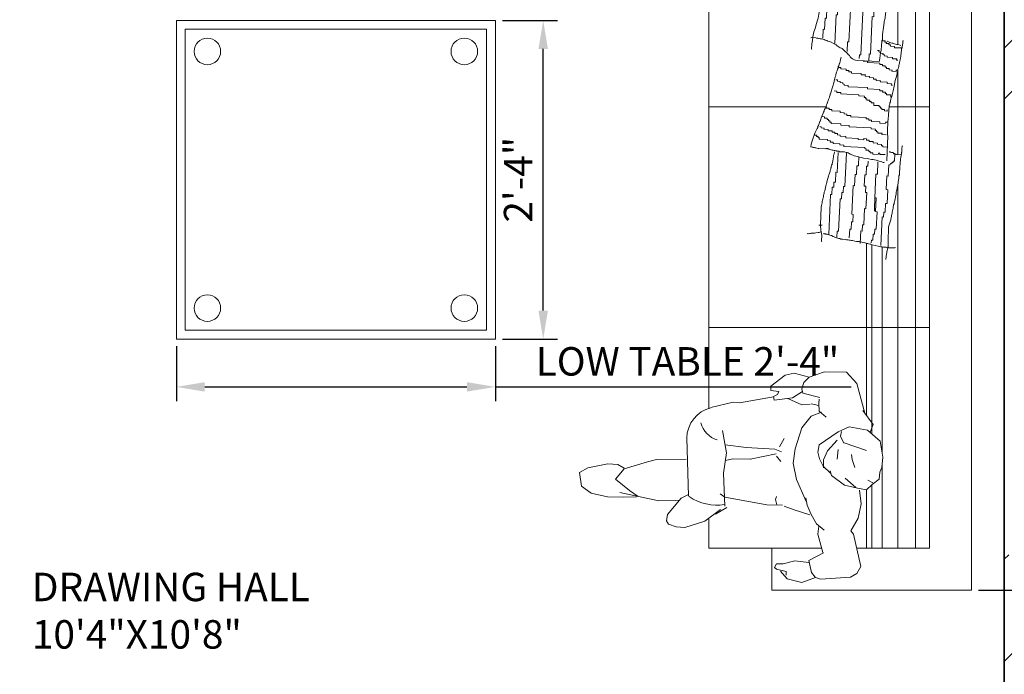
# Model space of a CAD drawing. Units: inches. Extents: x -138 to 270, y 8284 to 8764.
# Tile 7 of 10: x 112 to 198, y 8387 to 8444. Entities that reach past the tile are written whole.
import ezdxf

# ---------------------------------------------------------------- set-up
doc = ezdxf.new("R2010")
doc.units = ezdxf.units.IN
for name, color, linetype, lineweight in [('A-ANNO-DIMS', 2, 'Continuous', 18), ('A-AREA-IDEN', 7, 'Continuous', 18), ('FURNITURE', 8, 'Continuous', 15), ('FURNITURE1', 8, 'Continuous', 15), ('WALL', 8, 'Continuous', 35), ('WINDOW', 151, 'Continuous', 15)]:
    doc.layers.add(name, color=color, linetype=linetype, lineweight=lineweight)
doc.layers.add('A-WALL-PATT', color=32, linetype='Continuous', lineweight=9, true_color=0xbc761a)
doc.styles.get("Standard").update_dxf_attribs({"font": 'arial.ttf'})
doc.dimstyles.new('ISO-25', dxfattribs={"dimtxt": 2.5, "dimasz": 2.5, "dimexe": 1.25, "dimexo": 0.625, "dimtad": 1, "dimdec": 0, "dimlunit": 3, "dimtxsty": 'Standard', "dimcen": 2.5, "dimadec": 0, "dimazin": 0, "dimtfac": 1, "dimtdec": 0, "dimtmove": 0, "dimatfit": 3, "dimfxl": 1, "dimarcsym": 0})

# ---------------------------------------------------------------- blocks, each defined once
blk = doc.blocks.new('A$C48A43CE3')
at = {"layer": 'FURNITURE1', "ltscale": 2}
for p, q in [((21.39, 35.19), (21.36, 35.19)), ((21.42, 35.15), (21.39, 35.19)), ((21.68, 35.14), (21.42, 35.15)), ((21.74, 34.36), (21.64, 34.07)), ((21.77, 35.11), (21.68, 35.14)), ((21.77, 34.49), (21.74, 34.36)), ((21.88, 35.1), (21.77, 35.11)), ((21.78, 34.59), (21.77, 34.49)), ((21.84, 34.84), (21.78, 34.59)), ((21.88, 34.94), (21.84, 34.84)), ((22, 35.06), (21.88, 35.1)), ((22.18, 35.06), (22, 35.06)), ((22.16, 34.99), (22.13, 34.23)), ((22.23, 35.02), (22.18, 35.06)), ((22.49, 35.01), (22.23, 35.02)), ((22.58, 34.98), (22.49, 35.01)), ((22.79, 34.97), (22.58, 34.98)), ((22.9, 34.93), (22.79, 34.97)), ((23.08, 34.92), (22.9, 34.93)), ((23.25, 34.88), (23.08, 34.92)), ((23.45, 34.84), (23.25, 34.88)), ((23.36, 34.48), (23.34, 34.03)), ((23.5, 34.47), (23.36, 34.48)), ((23.6, 34.81), (23.45, 34.84)), ((23.5, 34.62), (23.5, 34.47)), ((23.71, 34.8), (23.6, 34.81)), ((23.77, 34.77), (23.71, 34.8)), ((23.95, 34.76), (23.77, 34.77)), ((24.03, 34.72), (23.95, 34.76)), ((24.18, 34.72), (24.03, 34.72)), ((24.32, 34.68), (24.18, 34.72)), ((24.41, 34.64), (24.32, 34.68)), ((24.52, 34.61), (24.41, 34.64)), ((24.64, 34.6), (24.52, 34.61)), ((24.59, 34.57), (24.58, 34.42)), ((24.58, 34.42), (24.72, 34.41)), ((24.73, 34.57), (24.64, 34.6)), ((24.72, 34.41), (24.69, 33.96)), ((24.84, 34.53), (24.73, 34.57)), ((24.96, 34.52), (24.84, 34.53)), ((25.1, 34.49), (24.96, 34.52)), ((25.28, 34.45), (25.1, 34.49)), ((25.48, 34.37), (25.28, 34.45)), ((25.71, 34.33), (25.48, 34.37)), ((26.32, 34.21), (25.71, 34.33)), ((33.66, 34.31), (33.53, 34.06)), ((33.72, 34.37), (33.66, 34.31)), ((33.68, 34.29), (33.67, 34.14)), ((34.49, 34.25), (33.68, 34.29)), ((33.75, 34.44), (33.72, 34.37)), ((33.74, 35.02), (33.77, 34.92)), ((33.77, 34.92), (33.75, 34.44)), ((34.48, 34.1), (34.49, 34.25)), ((14.06, 33.26), (13.66, 33.27)), ((14.06, 33.1), (14.06, 33.26)), ((21.4, 33.21), (21.38, 32.91)), ((21.53, 33.2), (21.4, 33.21)), ((21.57, 33.75), (21.41, 33.43)), ((21.54, 33.36), (21.53, 33.2)), ((21.68, 33.35), (21.54, 33.36)), ((21.63, 33.94), (21.57, 33.75)), ((21.64, 34.07), (21.63, 33.94)), ((21.69, 33.65), (21.68, 33.35)), ((21.83, 33.64), (21.69, 33.65)), ((21.83, 33.79), (21.83, 33.64)), ((21.97, 33.79), (21.83, 33.79)), ((21.99, 34.24), (21.97, 33.79)), ((22.13, 34.23), (21.99, 34.24)), ((23.04, 33.44), (23.02, 33.13)), ((23.17, 33.43), (23.04, 33.44)), ((23.2, 34.03), (23.17, 33.43)), ((23.34, 34.03), (23.2, 34.03)), ((24.12, 33.23), (24.1, 32.93)), ((24.25, 33.23), (24.12, 33.23)), ((24.26, 33.38), (24.25, 33.23)), ((24.39, 33.37), (24.26, 33.38)), ((24.41, 33.67), (24.39, 33.37)), ((24.54, 33.67), (24.41, 33.67)), ((24.56, 33.97), (24.54, 33.67)), ((24.69, 33.96), (24.56, 33.97)), ((25.89, 33.45), (25.86, 32.7)), ((26.03, 33.45), (25.89, 33.45)), ((26.05, 33.9), (26.03, 33.45)), ((26.19, 33.89), (26.05, 33.9)), ((26.19, 34.04), (26.19, 33.89)), ((26.49, 34.17), (26.32, 34.21)), ((26.64, 34.13), (26.49, 34.17)), ((26.81, 34.09), (26.64, 34.13)), ((27.1, 34.02), (26.81, 34.09)), ((26.97, 33.25), (26.96, 32.95)), ((27.11, 33.24), (26.97, 33.25)), ((27.21, 33.98), (27.1, 34.02)), ((27.11, 33.39), (27.11, 33.24)), ((27.25, 33.39), (27.11, 33.39)), ((27.33, 33.98), (27.21, 33.98)), ((27.27, 33.84), (27.25, 33.39)), ((27.54, 33.83), (27.27, 33.84)), ((27.42, 33.94), (27.33, 33.98)), ((27.48, 33.94), (27.42, 33.94)), ((27.56, 33.9), (27.48, 33.94)), ((27.62, 33.87), (27.56, 33.9)), ((27.71, 33.86), (27.62, 33.87)), ((27.94, 33.79), (27.71, 33.86)), ((28.02, 33.79), (27.94, 33.79)), ((28.14, 33.75), (28.02, 33.79)), ((28.26, 33.75), (28.14, 33.75)), ((28.34, 33.71), (28.26, 33.75)), ((28.46, 33.67), (28.34, 33.71)), ((28.66, 33.66), (28.46, 33.67)), ((28.78, 33.63), (28.66, 33.66)), ((29.62, 33.59), (28.78, 33.63)), ((28.88, 33.46), (29.02, 33.46)), ((29.02, 33.46), (29, 33.15)), ((29.77, 33.56), (29.62, 33.59)), ((29.94, 33.55), (29.77, 33.56)), ((30.12, 33.51), (29.94, 33.55)), ((31.23, 33.47), (30.12, 33.51)), ((30.24, 33.55), (30.23, 33.25)), ((30.23, 33.25), (30.37, 33.24)), ((30.37, 33.24), (30.34, 32.64)), ((31.34, 33.49), (31.23, 33.47)), ((31.61, 33.48), (31.34, 33.49)), ((31.59, 33.33), (31.57, 32.88)), ((31.72, 33.51), (31.61, 33.48)), ((34.44, 33.4), (31.72, 33.51)), ((32.96, 33.42), (32.93, 32.97)), ((33.46, 33.73), (33.45, 33.67)), ((33.49, 33.77), (33.46, 33.73)), ((33.52, 33.93), (33.49, 33.86)), ((33.49, 33.86), (33.49, 33.77)), ((33.53, 34.06), (33.52, 33.93)), ((33.67, 34.14), (33.53, 34.15)), ((33.76, 33.23), (33.73, 32.63)), ((34.62, 34.1), (34.48, 34.1)), ((34.61, 33.95), (34.62, 34.1)), ((34.75, 33.94), (34.61, 33.95)), ((34.74, 33.79), (34.75, 33.94)), ((34.88, 33.78), (34.74, 33.79)), ((34.87, 33.63), (34.88, 33.78)), ((36.09, 33.57), (34.87, 33.63)), ((36.08, 33.42), (36.09, 33.57)), ((37.57, 33.35), (36.08, 33.42)), ((37.58, 33.5), (37.57, 33.35)), ((39.07, 33.43), (37.58, 33.5)), ((39.06, 33.28), (39.07, 33.43)), ((40.01, 33.24), (39.06, 33.28)), ((40.01, 33.09), (40.01, 33.24)), ((12.33, 32.2), (12.24, 32.24)), ((12.45, 32.2), (12.33, 32.2)), ((12.59, 32.16), (12.45, 32.2)), ((12.73, 32.09), (12.59, 32.16)), ((14.87, 33.07), (14.06, 33.1)), ((14.86, 32.92), (14.87, 33.07)), ((15.68, 32.88), (14.86, 32.92)), ((15.67, 32.73), (15.68, 32.88)), ((16.08, 32.71), (15.67, 32.73)), ((16.07, 32.56), (16.08, 32.71)), ((16.75, 32.53), (16.07, 32.56)), ((16.74, 32.37), (16.75, 32.53)), ((17.15, 32.36), (16.74, 32.37)), ((17.14, 32.21), (17.15, 32.36)), ((17.68, 32.18), (17.14, 32.21)), ((17.67, 32.03), (17.68, 32.18)), ((22.45, 32.56), (22.45, 32.41)), ((22.59, 32.55), (22.45, 32.56)), ((22.6, 32.7), (22.59, 32.55)), ((22.73, 32.7), (22.6, 32.7)), ((22.75, 33), (22.73, 32.7)), ((22.88, 32.99), (22.75, 33)), ((22.89, 33.14), (22.88, 32.99)), ((23.02, 33.13), (22.89, 33.14)), ((23.62, 32.57), (23.52, 30.17)), ((23.82, 32.64), (23.75, 31.29)), ((23.95, 32.64), (23.82, 32.64)), ((23.97, 32.94), (23.95, 32.64)), ((24.1, 32.93), (23.97, 32.94)), ((25.56, 32.26), (25.55, 31.96)), ((25.7, 32.25), (25.56, 32.26)), ((25.72, 32.71), (25.7, 32.25)), ((25.86, 32.7), (25.72, 32.71)), ((26.67, 32.66), (26.61, 31.31)), ((26.81, 32.65), (26.67, 32.66)), ((26.82, 32.96), (26.81, 32.65)), ((26.96, 32.95), (26.82, 32.96)), ((28.43, 32.58), (28.4, 31.98)), ((28.57, 32.57), (28.43, 32.58)), ((28.58, 32.72), (28.57, 32.57)), ((28.71, 32.72), (28.58, 32.72)), ((28.72, 32.87), (28.71, 32.72)), ((28.85, 32.86), (28.72, 32.87)), ((28.87, 33.16), (28.85, 32.86)), ((29, 33.15), (28.87, 33.16)), ((30.2, 32.65), (30.16, 31.74)), ((30.34, 32.64), (30.2, 32.65)), ((30.99, 32.16), (30.97, 31.7)), ((31.13, 32.15), (30.99, 32.16)), ((31.14, 32.3), (31.13, 32.15)), ((31.27, 32.29), (31.14, 32.3)), ((31.28, 32.44), (31.27, 32.29)), ((31.42, 32.44), (31.28, 32.44)), ((31.44, 32.89), (31.42, 32.44)), ((31.57, 32.88), (31.44, 32.89)), ((32.5, 32.39), (32.48, 31.93)), ((32.64, 32.38), (32.5, 32.39)), ((32.66, 32.83), (32.64, 32.38)), ((32.79, 32.82), (32.66, 32.83)), ((32.8, 32.98), (32.79, 32.82)), ((32.93, 32.97), (32.8, 32.98)), ((33.6, 32.64), (33.59, 32.49)), ((33.59, 32.49), (33.73, 32.48)), ((33.73, 32.63), (33.6, 32.64)), ((33.73, 32.48), (33.7, 31.88)), ((34.4, 32.4), (34.29, 31.92)), ((34.46, 32.56), (34.4, 32.4)), ((34.5, 32.75), (34.46, 32.56)), ((34.56, 32.88), (34.5, 32.75)), ((35.9, 32.38), (34.54, 32.44)), ((34.6, 33.01), (34.56, 32.88)), ((34.57, 33.17), (34.6, 33.1)), ((34.6, 33.1), (34.6, 33.01)), ((35.89, 32.23), (35.9, 32.38)), ((38.46, 32.1), (35.89, 32.23)), ((38.2, 32.11), (39.91, 32.05)), ((38.47, 32.26), (38.46, 32.1)), ((39.96, 32.18), (38.47, 32.26)), ((39.97, 32.34), (39.96, 32.18)), ((41.87, 32.25), (39.97, 32.34)), ((40.55, 33.06), (40.01, 33.09)), ((40.54, 32.91), (40.55, 33.06)), ((43.66, 32.76), (40.54, 32.91)), ((41.86, 32.1), (41.87, 32.25)), ((11.81, 31.73), (11.75, 31.7)), ((11.9, 31.76), (11.81, 31.73)), ((11.93, 31.8), (11.9, 31.76)), ((11.99, 31.79), (11.93, 31.8)), ((12.02, 31.82), (11.99, 31.79)), ((12.14, 31.82), (12.02, 31.82)), ((12.2, 31.85), (12.14, 31.82)), ((12.43, 31.84), (12.2, 31.85)), ((12.58, 31.87), (12.43, 31.84)), ((12.72, 31.86), (12.58, 31.87)), ((12.87, 31.89), (12.72, 31.86)), ((12.91, 32.05), (12.73, 32.09)), ((12.99, 31.88), (12.87, 31.89)), ((13.02, 32.01), (12.91, 32.05)), ((13.11, 31.91), (12.99, 31.88)), ((13.25, 31.91), (13.11, 31.91)), ((13.32, 31.93), (13.19, 31.94)), ((13.31, 31.78), (13.32, 31.93)), ((14.13, 31.74), (13.31, 31.78)), ((14.12, 31.59), (14.13, 31.74)), ((14.53, 31.57), (14.12, 31.59)), ((14.52, 31.42), (14.53, 31.57)), ((14.79, 31.41), (14.52, 31.42)), ((14.78, 31.26), (14.79, 31.41)), ((15.46, 31.23), (14.78, 31.26)), ((15.46, 31.08), (15.46, 31.23)), ((16.4, 31.03), (15.46, 31.08)), ((18.76, 31.98), (17.67, 32.03)), ((18.75, 31.83), (18.76, 31.98)), ((22.82, 31.64), (18.75, 31.83)), ((22.81, 31.48), (22.82, 31.64)), ((23.62, 31.45), (22.81, 31.48)), ((23.62, 31.3), (23.6, 30.84)), ((23.75, 31.29), (23.62, 31.3)), ((25.1, 31.08), (25.08, 30.62)), ((25.24, 31.07), (25.1, 31.08)), ((25.26, 31.52), (25.24, 31.07)), ((25.39, 31.51), (25.26, 31.52)), ((25.42, 31.97), (25.39, 31.51)), ((25.55, 31.96), (25.42, 31.97)), ((26.47, 31.31), (26.37, 29.2)), ((26.61, 31.31), (26.47, 31.31)), ((27.55, 31.11), (27.54, 30.96)), ((27.68, 31.1), (27.55, 31.11)), ((27.69, 31.25), (27.68, 31.1)), ((27.83, 31.25), (27.69, 31.25)), ((27.84, 31.55), (27.83, 31.25)), ((27.98, 31.54), (27.84, 31.55)), ((27.98, 31.69), (27.98, 31.54)), ((28.12, 31.69), (27.98, 31.69)), ((28.13, 31.99), (28.12, 31.69)), ((28.4, 31.98), (28.13, 31.99)), ((29.72, 31.16), (29.65, 29.5)), ((29.86, 31.15), (29.72, 31.16)), ((29.87, 31.45), (29.86, 31.15)), ((30.01, 31.45), (29.87, 31.45)), ((30.02, 31.75), (30.01, 31.45)), ((30.16, 31.74), (30.02, 31.75)), ((30.84, 31.71), (30.72, 29.3)), ((30.97, 31.7), (30.84, 31.71)), ((32.04, 31.2), (32.02, 30.9)), ((32.17, 31.19), (32.04, 31.2)), ((32.19, 31.5), (32.17, 31.19)), ((32.32, 31.49), (32.19, 31.5)), ((32.34, 31.94), (32.32, 31.49)), ((32.48, 31.93), (32.34, 31.94)), ((33.12, 31.15), (33.11, 31)), ((33.26, 31.14), (33.12, 31.15)), ((33.27, 31.44), (33.26, 31.14)), ((33.41, 31.44), (33.27, 31.44)), ((33.41, 31.59), (33.41, 31.44)), ((33.55, 31.58), (33.41, 31.59)), ((33.56, 31.88), (33.55, 31.58)), ((33.7, 31.88), (33.56, 31.88)), ((34.2, 31.27), (34.13, 30.88)), ((34.21, 31.43), (34.2, 31.27)), ((34.28, 31.75), (34.21, 31.43)), ((34.29, 31.92), (34.28, 31.75)), ((35.03, 31.36), (34.49, 31.39)), ((35.03, 31.21), (35.03, 31.36)), ((35.97, 31.17), (35.03, 31.21)), ((35.97, 31.02), (35.97, 31.17)), ((37.19, 31.11), (37.19, 30.96)), ((37.87, 31.08), (37.19, 31.11)), ((37.88, 31.23), (37.87, 31.08)), ((39.64, 31.14), (37.88, 31.23)), ((39.02, 31.23), (39.02, 31.23)), ((39.63, 30.99), (39.64, 31.14)), ((42.4, 32.07), (41.86, 32.1)), ((42.4, 31.92), (42.4, 32.07)), ((43.07, 31.89), (42.4, 31.92)), ((43.07, 31.74), (43.07, 31.89)), ((43.34, 31.72), (43.07, 31.74)), ((13.41, 30.87), (13, 30.89)), ((13.4, 30.72), (13.41, 30.87)), ((13.81, 30.7), (13.4, 30.72)), ((13.8, 30.55), (13.81, 30.7)), ((14.34, 30.53), (13.8, 30.55)), ((14.34, 30.38), (14.34, 30.53)), ((14.74, 30.36), (14.34, 30.38)), ((14.73, 30.21), (14.74, 30.36)), ((14.87, 30.2), (14.73, 30.21)), ((14.86, 30.05), (14.87, 30.2)), ((15.13, 30.04), (14.86, 30.05)), ((15.13, 29.89), (15.13, 30.04)), ((16.4, 30.88), (16.4, 31.03)), ((22.9, 30.58), (16.4, 30.88)), ((22.9, 30.42), (22.9, 30.58)), ((23.3, 30.41), (22.9, 30.42)), ((23.49, 30.01), (23.45, 29.88)), ((23.52, 30.17), (23.49, 30.01)), ((24.94, 30.63), (24.89, 29.58)), ((25.08, 30.62), (24.94, 30.63)), ((27.24, 30.37), (27.15, 28.41)), ((27.38, 30.36), (27.24, 30.37)), ((27.41, 30.97), (27.38, 30.36)), ((27.54, 30.96), (27.41, 30.97)), ((31.99, 30.3), (31.93, 28.94)), ((32.13, 30.29), (31.99, 30.3)), ((32.02, 30.9), (32.16, 30.89)), ((32.16, 30.89), (32.13, 30.29)), ((32.98, 31.01), (32.87, 28.75)), ((33.11, 31), (32.98, 31.01)), ((33.92, 30.02), (33.88, 29.85)), ((33.98, 30.21), (33.92, 30.02)), ((34.02, 30.43), (33.98, 30.21)), ((34.09, 30.66), (34.02, 30.43)), ((34.85, 30.31), (34.03, 30.35)), ((34.13, 30.88), (34.09, 30.66)), ((34.71, 30.32), (34.85, 30.31)), ((34.98, 30.31), (34.71, 30.32)), ((34.98, 30.16), (34.98, 30.31)), ((35.92, 30.11), (34.98, 30.16)), ((35.92, 29.96), (35.92, 30.11)), ((37.19, 30.96), (35.97, 31.02)), ((41.4, 30.91), (39.63, 30.99)), ((41.39, 30.76), (41.4, 30.91)), ((42.07, 30.73), (41.39, 30.76)), ((42.06, 30.58), (42.07, 30.73)), ((43.42, 30.51), (42.06, 30.58)), ((12.53, 29.56), (12.54, 29.71)), ((13.07, 29.53), (12.53, 29.56)), ((12.54, 29.71), (12.67, 29.7)), ((13.07, 29.38), (13.07, 29.53)), ((14.15, 29.33), (13.07, 29.38)), ((14.14, 29.18), (14.15, 29.33)), ((15.63, 29.11), (14.14, 29.18)), ((15.53, 29.87), (15.13, 29.89)), ((15.53, 29.72), (15.53, 29.87)), ((17.29, 29.63), (15.53, 29.72)), ((15.63, 28.96), (15.63, 29.11)), ((15.9, 28.94), (15.63, 28.96)), ((15.89, 28.79), (15.9, 28.94)), ((17.28, 29.48), (17.29, 29.63)), ((21.48, 29.28), (17.28, 29.48)), ((21.48, 29.13), (21.48, 29.28)), ((22.56, 29.08), (21.48, 29.13)), ((22.57, 28.91), (22.23, 28.56)), ((22.66, 29.03), (22.57, 28.91)), ((22.75, 29.13), (22.66, 29.03)), ((22.87, 29.22), (22.75, 29.13)), ((22.99, 29.34), (22.87, 29.22)), ((23.14, 29.44), (22.99, 29.34)), ((23.23, 29.53), (23.14, 29.44)), ((23.33, 29.66), (23.23, 29.53)), ((23.39, 29.75), (23.33, 29.66)), ((23.45, 29.88), (23.39, 29.75)), ((24.46, 28.99), (24.43, 28.39)), ((24.6, 28.99), (24.46, 28.99)), ((24.61, 29.29), (24.6, 28.99)), ((24.75, 29.28), (24.61, 29.29)), ((24.76, 29.58), (24.75, 29.28)), ((24.89, 29.58), (24.76, 29.58)), ((26.24, 29.21), (26.22, 28.76)), ((26.37, 29.2), (26.24, 29.21)), ((29.35, 29.06), (29.34, 28.76)), ((29.49, 29.06), (29.35, 29.06)), ((29.51, 29.51), (29.49, 29.06)), ((29.65, 29.5), (29.51, 29.51)), ((30.59, 29.31), (30.55, 28.4)), ((30.72, 29.3), (30.59, 29.31)), ((31.79, 28.95), (31.77, 28.35)), ((31.93, 28.94), (31.79, 28.95)), ((33.52, 28.99), (33.46, 28.8)), ((33.53, 29.09), (33.52, 28.99)), ((33.56, 29.19), (33.53, 29.09)), ((33.63, 29.31), (33.56, 29.19)), ((37.22, 28.84), (33.56, 29.02)), ((33.69, 29.38), (33.63, 29.31)), ((33.72, 29.44), (33.69, 29.38)), ((33.75, 29.53), (33.72, 29.44)), ((33.78, 29.6), (33.75, 29.53)), ((33.82, 29.73), (33.78, 29.6)), ((33.88, 29.85), (33.82, 29.73)), ((37.14, 29.9), (35.92, 29.96)), ((37.13, 29.75), (37.14, 29.9)), ((40.25, 29.61), (37.13, 29.75)), ((40.26, 29.76), (40.25, 29.61)), ((41.07, 29.72), (40.26, 29.76)), ((41.06, 29.57), (41.07, 29.72)), ((41.88, 29.53), (41.06, 29.57)), ((41.87, 29.38), (41.88, 29.53)), ((42.82, 29.33), (41.87, 29.38)), ((12.08, 28.67), (12.22, 28.67)), ((12.22, 28.67), (12.08, 28.67)), ((12.21, 28.51), (12.22, 28.67)), ((13.43, 28.46), (12.21, 28.51)), ((13.42, 28.31), (13.43, 28.46)), ((13.96, 28.28), (13.42, 28.31)), ((13.96, 28.13), (13.96, 28.28)), ((15.18, 28.07), (13.96, 28.13)), ((15.17, 27.92), (15.18, 28.07)), ((15.31, 27.92), (15.17, 27.92)), ((15.3, 27.77), (15.31, 27.92)), ((16.16, 28.78), (15.89, 28.79)), ((16.16, 28.63), (16.16, 28.78)), ((16.29, 28.62), (16.16, 28.63)), ((16.28, 28.47), (16.29, 28.62)), ((16.55, 28.46), (16.28, 28.47)), ((16.55, 28.31), (16.55, 28.46)), ((17.23, 28.28), (16.55, 28.31)), ((17.22, 28.13), (17.23, 28.28)), ((18.57, 28.06), (17.22, 28.13)), ((18.57, 27.91), (18.57, 28.06)), ((21.68, 27.77), (18.57, 27.91)), ((21.82, 27.9), (21.76, 27.77)), ((21.92, 28.02), (21.82, 27.9)), ((22.01, 28.12), (21.92, 28.02)), ((22.07, 28.24), (22.01, 28.12)), ((22.13, 28.34), (22.07, 28.24)), ((22.17, 28.47), (22.13, 28.34)), ((22.23, 28.56), (22.17, 28.47)), ((23.22, 28.39), (23.16, 28.43)), ((23.48, 28.38), (23.22, 28.39)), ((23.57, 28.35), (23.48, 28.38)), ((23.68, 28.34), (23.57, 28.35)), ((23.74, 28.31), (23.68, 28.34)), ((23.8, 28.31), (23.74, 28.31)), ((23.82, 28.27), (23.8, 28.31)), ((23.88, 28.27), (23.82, 28.27)), ((23.91, 28.24), (23.88, 28.27)), ((23.97, 28.23), (23.91, 28.24)), ((24.03, 28.2), (23.97, 28.23)), ((24.11, 28.2), (24.03, 28.2)), ((24.14, 28.16), (24.11, 28.2)), ((24.2, 28.16), (24.14, 28.16)), ((24.28, 28.1), (24.15, 28.1)), ((24.26, 28.13), (24.2, 28.16)), ((24.34, 28.12), (24.26, 28.13)), ((24.3, 28.4), (24.28, 28.1)), ((24.43, 28.39), (24.3, 28.4)), ((24.46, 28.05), (24.34, 28.12)), ((24.52, 28.05), (24.46, 28.05)), ((24.57, 28.02), (24.52, 28.05)), ((24.63, 28.01), (24.57, 28.02)), ((24.8, 27.94), (24.63, 28.01)), ((25.04, 27.87), (24.8, 27.94)), ((25.15, 27.86), (25.04, 27.87)), ((25.24, 27.83), (25.15, 27.86)), ((25.64, 28.03), (25.63, 27.88)), ((25.77, 28.03), (25.64, 28.03)), ((25.79, 28.33), (25.77, 28.03)), ((25.92, 28.32), (25.79, 28.33)), ((25.94, 28.62), (25.92, 28.32)), ((26.07, 28.62), (25.94, 28.62)), ((26.08, 28.77), (26.07, 28.62)), ((26.22, 28.76), (26.08, 28.77)), ((26.86, 27.97), (26.84, 27.67)), ((26.99, 27.97), (26.86, 27.97)), ((27.01, 28.42), (26.99, 27.97)), ((27.15, 28.41), (27.01, 28.42)), ((29.05, 28.32), (29, 27.42)), ((29.18, 28.32), (29.05, 28.32)), ((29.2, 28.77), (29.18, 28.32)), ((29.34, 28.76), (29.2, 28.77)), ((30.41, 28.41), (30.36, 27.36)), ((30.55, 28.4), (30.41, 28.41)), ((31.48, 28.06), (31.47, 27.76)), ((31.62, 28.05), (31.48, 28.06)), ((31.63, 28.35), (31.62, 28.05)), ((31.77, 28.35), (31.63, 28.35)), ((32.58, 28.31), (32.54, 27.56)), ((32.71, 28.3), (32.58, 28.31)), ((32.74, 28.75), (32.71, 28.3)), ((32.87, 28.75), (32.74, 28.75)), ((33.36, 27.86), (33.3, 27.74)), ((33.39, 27.96), (33.36, 27.93)), ((33.36, 27.93), (33.36, 27.86)), ((33.4, 28.19), (33.39, 27.96)), ((33.44, 28.25), (33.4, 28.19)), ((33.46, 28.8), (33.44, 28.25)), ((35.69, 28.01), (33.52, 28.11)), ((35.68, 27.86), (35.69, 28.01)), ((36.77, 27.81), (35.68, 27.86)), ((37.22, 28.69), (37.22, 28.84)), ((37.89, 28.66), (37.22, 28.69)), ((37.89, 28.51), (37.89, 28.66)), ((38.57, 28.48), (37.89, 28.51)), ((38.56, 28.33), (38.57, 28.48)), ((42.08, 28.16), (38.56, 28.33)), ((42.08, 28.01), (42.08, 28.16)), ((42.75, 27.98), (42.08, 28.01)), ((15.84, 27.74), (15.3, 27.77)), ((15.83, 27.59), (15.84, 27.74)), ((16.38, 27.56), (15.83, 27.59)), ((16.37, 27.41), (16.38, 27.56)), ((16.78, 27.39), (16.37, 27.41)), ((16.77, 27.24), (16.78, 27.39)), ((17.04, 27.23), (16.77, 27.24)), ((17.03, 27.08), (17.04, 27.23)), ((17.85, 27.04), (17.03, 27.08)), ((17.84, 26.89), (17.85, 27.04)), ((18.92, 26.84), (17.84, 26.89)), ((18.92, 26.69), (18.92, 26.84)), ((21.34, 26.88), (21.31, 26.72)), ((21.41, 27.01), (21.34, 26.88)), ((21.44, 27.13), (21.41, 27.01)), ((21.51, 27.29), (21.44, 27.13)), ((21.7, 27.68), (21.51, 27.29)), ((21.76, 27.77), (21.7, 27.68)), ((25.3, 27.79), (25.24, 27.83)), ((25.35, 27.79), (25.3, 27.79)), ((25.44, 27.75), (25.35, 27.79)), ((25.58, 27.72), (25.44, 27.75)), ((25.76, 27.68), (25.58, 27.72)), ((25.96, 27.64), (25.76, 27.68)), ((26.31, 27.53), (25.96, 27.64)), ((26.54, 27.48), (26.31, 27.53)), ((26.88, 27.37), (26.54, 27.48)), ((27.06, 27.33), (26.88, 27.37)), ((27.14, 27.3), (27.06, 27.33)), ((27.2, 27.26), (27.14, 27.3)), ((27.26, 27.26), (27.2, 27.26)), ((27.35, 27.22), (27.26, 27.26)), ((27.46, 27.19), (27.35, 27.22)), ((27.61, 27.15), (27.46, 27.19)), ((27.75, 27.08), (27.61, 27.15)), ((27.98, 27), (27.75, 27.08)), ((28.07, 26.97), (27.98, 27)), ((28.12, 26.97), (28.07, 26.97)), ((28.15, 26.93), (28.12, 26.97)), ((28.21, 26.93), (28.15, 26.93)), ((28.27, 26.9), (28.21, 26.93)), ((28.35, 26.86), (28.27, 26.9)), ((28.5, 26.82), (28.35, 26.86)), ((28.61, 26.78), (28.5, 26.82)), ((28.71, 26.83), (28.57, 26.84)), ((28.76, 26.71), (28.61, 26.78)), ((28.72, 27.13), (28.71, 26.83)), ((28.86, 27.13), (28.72, 27.13)), ((28.87, 27.43), (28.86, 27.13)), ((29, 27.42), (28.87, 27.43)), ((29.8, 26.93), (29.78, 26.63)), ((29.93, 26.92), (29.8, 26.93)), ((29.94, 27.07), (29.93, 26.92)), ((30.08, 27.07), (29.94, 27.07)), ((30.08, 27.22), (30.08, 27.07)), ((30.22, 27.21), (30.08, 27.22)), ((30.23, 27.36), (30.22, 27.21)), ((30.36, 27.36), (30.23, 27.36)), ((31.02, 27.02), (31, 26.57)), ((31.16, 27.02), (31.02, 27.02)), ((31.18, 27.47), (31.16, 27.02)), ((31.32, 27.46), (31.18, 27.47)), ((31.33, 27.76), (31.32, 27.46)), ((31.47, 27.76), (31.33, 27.76)), ((32.11, 26.97), (32.07, 26.07)), ((32.24, 26.97), (32.11, 26.97)), ((32.26, 27.27), (32.24, 26.97)), ((32.39, 27.26), (32.26, 27.27)), ((32.41, 27.56), (32.39, 27.26)), ((32.54, 27.56), (32.41, 27.56)), ((33.12, 27), (33.09, 26.96)), ((33.09, 26.96), (33.09, 26.83)), ((33.09, 26.83), (33.14, 26.77)), ((33.14, 26.77), (33.11, 26.02)), ((33.16, 27.12), (33.12, 27.06)), ((33.12, 27.06), (33.12, 27)), ((33.26, 27.48), (33.16, 27.19)), ((33.16, 27.19), (33.16, 27.12)), ((33.3, 27.67), (33.26, 27.57)), ((33.26, 27.57), (33.26, 27.48)), ((33.3, 27.74), (33.3, 27.67)), ((36.76, 27.66), (36.77, 27.81)), ((37.3, 27.63), (36.76, 27.66)), ((37.3, 27.48), (37.3, 27.63)), ((38.11, 27.44), (37.3, 27.48)), ((38.1, 27.29), (38.11, 27.44)), ((42.44, 27.09), (38.1, 27.29)), ((20.14, 26.63), (18.92, 26.69)), ((20.13, 26.48), (20.14, 26.63)), ((21.08, 26.44), (20.13, 26.48)), ((21.09, 25.75), (21.06, 25.69)), ((21.1, 25.91), (21.09, 25.75)), ((21.13, 25.98), (21.1, 25.91)), ((21.17, 26.17), (21.13, 26.07)), ((21.13, 26.07), (21.13, 25.98)), ((21.21, 26.46), (21.17, 26.3)), ((21.17, 26.3), (21.17, 26.17)), ((21.24, 26.59), (21.21, 26.46)), ((21.31, 26.72), (21.24, 26.59)), ((28.87, 26.64), (28.76, 26.71)), ((28.96, 26.61), (28.87, 26.64)), ((29.02, 26.61), (28.96, 26.61)), ((29.13, 26.54), (29.02, 26.61)), ((29.24, 26.5), (29.13, 26.54)), ((29.76, 26.28), (29.24, 26.5)), ((29.65, 26.64), (29.63, 26.34)), ((29.78, 26.63), (29.65, 26.64)), ((29.91, 26.25), (29.76, 26.28)), ((30.02, 26.21), (29.91, 26.25)), ((30.11, 26.17), (30.02, 26.21)), ((30.16, 26.14), (30.11, 26.17)), ((30.25, 26.1), (30.16, 26.14)), ((30.6, 25.99), (30.25, 26.1)), ((30.71, 25.92), (30.6, 25.99)), ((30.72, 26.28), (30.71, 26.13)), ((30.8, 25.89), (30.71, 25.92)), ((30.85, 26.28), (30.72, 26.28)), ((30.91, 25.85), (30.8, 25.89)), ((30.87, 26.58), (30.85, 26.28)), ((31, 26.57), (30.87, 26.58)), ((31, 25.81), (30.91, 25.85)), ((31.08, 25.75), (31, 25.81)), ((31.37, 25.6), (31.08, 25.75)), ((31.65, 25.79), (31.63, 25.49)), ((31.78, 25.78), (31.65, 25.79)), ((31.79, 25.93), (31.78, 25.78)), ((31.92, 25.93), (31.79, 25.93)), ((31.93, 26.08), (31.92, 25.93)), ((32.07, 26.07), (31.93, 26.08)), ((33.07, 25.8), (33.04, 25.7)), ((33.04, 25.7), (33.04, 25.64)), ((33.08, 25.96), (33.07, 25.8)), ((33.11, 26.02), (33.08, 25.96)), ((41.44, 26.02), (41.45, 26.37)), ((42.17, 26.18), (42.23, 26.05)), ((42.23, 26.05), (42.22, 25.95)), ((42.22, 25.95), (42.27, 25.69)), ((42.27, 25.69), (42.29, 25.53)), ((21.06, 25.69), (21.04, 25.23)), ((21.04, 25.23), (21.07, 25.14)), ((31.54, 25.56), (31.37, 25.6)), ((31.66, 25.5), (31.54, 25.56)), ((31.92, 25.39), (31.66, 25.5)), ((31.97, 25.39), (31.92, 25.39)), ((32.15, 25.31), (31.97, 25.39)), ((32.61, 25.17), (32.15, 25.31)), ((32.9, 25.15), (32.61, 25.17)), ((32.93, 25.19), (32.9, 25.15)), ((32.94, 25.35), (32.93, 25.19)), ((32.97, 25.38), (32.94, 25.35)), ((33, 25.54), (32.97, 25.48)), ((32.97, 25.48), (32.97, 25.38)), ((33.01, 25.6), (33, 25.54)), ((33.04, 25.64), (33.01, 25.6)), ((42.29, 25.53), (42.29, 25.37)), ((42.29, 25.37), (42.31, 25.2)), ((42.31, 25.2), (42.33, 25.1)), ((42.33, 25.1), (42.33, 25.01)), ((42.33, 25.01), (42.36, 24.94)), ((42.36, 24.94), (42.35, 24.81)), ((42.35, 24.81), (42.38, 24.75))]:
    blk.add_line(p, q, dxfattribs=at)
at = {"layer": 'FURNITURE1'}
for p, q in [((63.73, 31.32), (64.91, 32.67)), ((64.91, 32.67), (66.68, 32.96)), ((66.68, 32.96), (67.78, 32.88)), ((67.78, 32.88), (68.31, 32.65)), ((68.31, 32.65), (69.04, 32.56)), ((69.04, 32.56), (69.62, 31.81)), ((61.6, 30.79), (63.12, 31.91)), ((63.12, 31.91), (63.95, 31.58)), ((63.37, 29.3), (63.73, 31.32)), ((65.11, 28.76), (65.94, 31.18)), ((69.47, 31.89), (69.17, 31.35)), ((69.62, 31.81), (70.21, 31.21)), ((70.21, 31.21), (70.04, 30.22)), ((57.41, 29.03), (58.64, 30.16)), ((58.64, 30.16), (61.89, 31)), ((68.95, 28.88), (69.95, 30.05)), ((70.04, 30.22), (69.71, 28.81)), ((71.74, 30.63), (70.26, 30.44)), ((73.3, 30.29), (71.74, 30.63)), ((74.67, 29.49), (73.3, 30.29)), ((78.55, 30.57), (75.04, 29.77)), ((79.32, 30.14), (78.55, 30.57)), ((79.72, 29.45), (79.32, 30.14)), ((57.39, 26.62), (57.41, 29.03)), ((63.91, 28.1), (63.37, 29.3)), ((66.93, 29.65), (66.38, 29.55)), ((67.79, 29.92), (66.93, 29.65)), ((75.04, 29.77), (74.67, 29.49)), ((79.92, 26.2), (79.72, 29.45)), ((64.38, 28.38), (63.87, 28.49)), ((65.34, 26.06), (63.91, 28.1)), ((65.13, 28.73), (64.38, 28.38)), ((65.97, 26.96), (64.81, 28.02)), ((66.87, 28.02), (65.83, 28.12)), ((69.71, 28.81), (68.66, 27.41)), ((62.32, 26.83), (61.66, 26.07)), ((66.97, 26.54), (65.97, 26.96)), ((68.4, 27.27), (67.64, 26.48)), ((68.66, 27.41), (68.16, 27.24)), ((57.95, 24.98), (57.39, 26.62)), ((60.16, 26.13), (59.71, 24.29)), ((60.84, 26.02), (60.36, 26.06)), ((61.66, 26.07), (60.84, 26.02)), ((61.03, 26.03), (60.86, 25.18)), ((62.21, 25.2), (61.78, 26.32)), ((66.12, 25.9), (65.34, 26.06)), ((66.86, 26.1), (66.12, 25.9)), ((67.64, 26.48), (66.86, 26.1)), ((67.84, 26.53), (66.97, 26.54)), ((73.91, 25.77), (72.91, 25.18)), ((74.59, 26.61), (73.91, 25.77)), ((75.03, 25.92), (74.16, 26.01)), ((77.02, 26.46), (75.03, 25.92)), ((77.92, 24.92), (77.07, 26.52)), ((79.75, 25.65), (79.92, 26.2)), ((57.54, 23.33), (57.95, 24.98)), ((57.95, 24.98), (58.54, 24.37)), ((60.9, 25.08), (60.98, 24.17)), ((63.49, 24.17), (62.21, 25.2)), ((71.49, 24.63), (69.1, 23.59)), ((71.89, 24.73), (71.1, 24.59)), ((72.91, 25.18), (71.89, 24.73)), ((72.38, 23.32), (72.95, 25.03)), ((79.2, 25.21), (77.92, 24.92)), ((78.13, 24.93), (77.95, 23.41)), ((79.7, 25.63), (79.2, 25.21)), ((80.29, 24.17), (79.75, 25.65)), ((58.54, 24.37), (59.25, 24.18)), ((59.25, 24.18), (59.71, 24.29)), ((59.52, 24.23), (60.23, 23.17)), ((60.98, 24.17), (60.29, 22.63)), ((65.75, 23.44), (63.49, 24.17)), ((69.1, 23.59), (67.32, 23.24)), ((79.9, 22.59), (80.29, 24.17)), ((57.73, 22.35), (57.54, 23.33)), ((60.23, 23.17), (60.45, 21.16)), ((67.32, 23.24), (65.75, 23.44)), ((72.01, 22.25), (72.38, 23.32)), ((77.95, 23.41), (78.27, 22.14)), ((78.86, 21.4), (79.09, 22.48)), ((79.08, 21.86), (79.9, 22.59)), ((79.09, 22.48), (79.5, 22.45)), ((58.93, 20.81), (57.73, 22.35)), ((59.54, 21.67), (59.4, 20.81)), ((59.85, 21.53), (59.54, 21.67)), ((60.06, 21.08), (59.85, 21.53)), ((64.63, 22.24), (65.53, 21.74)), ((65.8, 21.23), (66.09, 21.96)), ((66.56, 21.41), (67.13, 21.88)), ((71.27, 21.29), (70.94, 21.43)), ((71.86, 21.46), (71.27, 21.29)), ((71.86, 20.35), (71.89, 22.08)), ((78.27, 22.14), (78.25, 21.41)), ((59.4, 20.81), (58.93, 20.81)), ((60.45, 21.16), (60.06, 21.08)), ((60.12, 21.08), (60.74, 17.4)), ((65.61, 18.12), (65.8, 21.23)), ((66.32, 21.37), (66.87, 18.56)), ((71.03, 15.78), (71.86, 20.35)), ((78.25, 21.41), (78.68, 21.2)), ((78.86, 21.4), (78.68, 21.2)), ((66.87, 18.6), (66.86, 16.67)), ((60.74, 17.4), (60.69, 16.7)), ((65.32, 15.82), (65.61, 18.12)), ((60.69, 16.7), (61.28, 14.28)), ((66.86, 16.67), (67.01, 15.86)), ((66.19, 15.98), (63.76, 15.54)), ((68.41, 15.66), (66.19, 15.98)), ((72.01, 15.78), (68.41, 15.66)), ((70.64, 15.3), (71.03, 15.78)), ((71, 15.74), (70.99, 15.79)), ((72.87, 14.79), (72.13, 16.01)), ((73.63, 13.63), (72.35, 15.33)), ((74.3, 11.44), (73.63, 13.63)), ((64.58, 11.65), (70.9, 11.84)), ((70.71, 11.83), (71.14, 11.05)), ((66.91, 8.38), (66.88, 11.59)), ((71.14, 11.05), (72.9, 9.56)), ((71.36, 10.43), (71.33, 10.9)), ((74.23, 10.49), (74.3, 11.44)), ((71.42, 8.64), (71.36, 10.43)), ((73.59, 9.44), (73.96, 9.67)), ((73.96, 9.67), (74.23, 10.49)), ((70.49, 4.37), (71.42, 8.64)), ((72.9, 9.56), (73.59, 9.44)), ((66.91, 8.38), (67.17, 7.38)), ((67.17, 7.38), (67.94, 4.86)), ((69.04, 3.92), (70.29, 5.44)), ((70.29, 5.44), (70.93, 6.37)), ((71.03, 4.82), (70.97, 6.18)), ((67.85, 4.84), (67.47, 4.16)), ((67.94, 4.86), (69.04, 3.92)), ((70.99, 3.03), (71.03, 4.82)), ((67.47, 4.16), (67.39, 3.07)), ((67.39, 3.07), (67.84, 0.9)), ((70.57, 1.26), (70.99, 3.03)), ((69.82, 0.2), (70.57, 1.26)), ((67.84, 0.9), (68.34, 0)), ((68.34, 0), (69.82, 0.2))]:
    blk.add_line(p, q, dxfattribs=at)
for points in [[(76.57, 20.9), (81.14, 20.9), (81.14, 42.62), (0, 42.62), (0, 20.9), (4.57, 20.9)], [(61.35, 14.04), (4.57, 14.04), (4.57, 38.04), (76.57, 38.04), (76.57, 30.12)], [(4.57, 14.04), (4.57, 38.04)], [(28.57, 33.67), (28.57, 38.04)], [(52.57, 14.04), (52.57, 38.04)], [(76.57, 36.51), (4.57, 36.51)], [(21.78, 34.62), (4.57, 34.62)], [(33.76, 34.62), (24.5, 34.62)], [(76.57, 34.62), (36.97, 34.62)], [(13.35, 32.9), (4.57, 32.9)], [(66.32, 32.9), (43.79, 32.9)], [(76.57, 32.9), (67.44, 32.9)], [(13.07, 31.76), (4.57, 31.76)], [(12.99, 31.19), (4.57, 31.19)], [(62.14, 31.19), (43.41, 31.19)], [(64.11, 31.76), (43.55, 31.76)], [(63.49, 31.76), (64.11, 31.76)], [(64.11, 31.76), (63.49, 31.76)], [(76.57, 31.76), (69.66, 31.76)], [(76.57, 31.19), (70.21, 31.19)], [(28.57, 14.04), (28.57, 26.8)], [(76.57, 26.34), (76.57, 14.04), (73.31, 14.04)]]:
    blk.add_lwpolyline(points, dxfattribs=at)
at = {"layer": 'FURNITURE1', "ltscale": 2}
for points in [[(13.77, 35.36), (13.83, 35.29), (13.83, 35.23), (13.85, 35.16), (13.83, 34.71), (13.8, 34.51), (13.79, 34.35), (13.68, 33.87), (13.68, 33.74), (13.61, 33.61), (13.55, 33.35), (13.48, 33.26), (13.45, 33.13), (13.38, 33), (13.32, 32.81), (13.28, 32.68), (13.25, 32.62), (13.12, 32.23), (13.12, 32.14), (13.08, 32.01), (13.07, 31.75), (13.03, 31.59), (13.03, 31.43), (12.99, 31.27), (12.99, 31.14), (12.95, 30.98), (12.92, 30.88), (12.91, 30.78), (12.88, 30.72), (12.88, 30.65), (12.85, 30.59), (12.81, 30.49), (12.81, 30.43), (12.78, 30.33), (12.77, 30.14), (12.74, 30.04), (12.68, 28.75), (12.65, 28.68), (12.62, 28.59), (12.56, 28.46), (12.55, 28.39), (12.52, 28.33), (12.49, 28.23), (12.48, 28.04), (12.45, 28.01)], [(23.59, 32.6), (23.48, 32.6), (23.3, 32.64), (22.95, 32.69), (22.72, 32.73), (22.4, 32.78), (22.23, 32.78), (22.08, 32.82), (21.76, 32.83), (21.65, 32.87), (21.38, 32.88), (21.27, 32.92), (20.66, 32.94), (20.48, 32.98), (20.13, 33), (19.99, 33.03), (19.87, 33.04), (19.76, 33.08), (19.58, 33.08), (19.47, 33.12), (19.29, 33.13), (19.12, 33.17), (18.91, 33.21), (18.74, 33.21), (18.57, 33.25), (18.42, 33.26), (18.25, 33.3), (18.1, 33.34), (17.9, 33.41), (17.73, 33.45), (17.55, 33.52), (17.41, 33.59), (17.27, 33.63), (17.12, 33.7), (16.89, 33.77), (16.75, 33.81), (16.58, 33.88), (16.37, 33.92), (16.14, 34), (15.94, 34.07), (15.8, 34.14), (15.68, 34.18), (15.62, 34.18), (15.57, 34.22), (15.48, 34.22), (15.25, 34.29), (15.08, 34.33), (14.93, 34.34), (14.81, 34.38), (14.76, 34.38), (14.7, 34.41), (14.55, 34.42), (14.47, 34.45), (14.15, 34.47), (14.09, 34.5), (13.91, 34.51), (13.83, 34.54), (13.74, 34.55), (13.39, 34.66), (13.28, 34.73), (13.22, 34.73), (13.19, 34.76)], [(45.18, 33.3), (44.83, 33.32), (44.37, 33.4), (44.2, 33.44), (44.05, 33.48), (43.96, 33.48), (43.91, 33.51), (43.82, 33.52), (43.79, 33.55), (43.3, 33.57), (43.21, 33.54), (41.63, 33.6), (41.52, 33.64), (41.08, 33.76), (40.85, 33.83), (40.76, 33.83), (40.68, 33.87), (40.59, 33.87), (40.48, 33.91), (40.39, 33.91), (40.27, 33.95), (40.13, 33.99), (40.01, 33.99), (39.72, 34.07), (39.58, 34.08), (39.43, 34.11), (39.32, 34.15), (39.23, 34.15), (39.11, 34.19), (39, 34.2), (38.88, 34.23), (38.74, 34.27), (38.56, 34.31), (38.36, 34.35), (38.01, 34.43), (37.84, 34.44), (37.69, 34.47), (37.58, 34.48), (37.43, 34.52), (37.32, 34.52), (37.2, 34.56), (37.06, 34.6), (36.88, 34.64), (36.71, 34.64), (36.36, 34.72), (36.07, 34.73), (35.95, 34.77), (34.99, 34.81), (34.85, 34.85), (34.55, 34.86), (34.44, 34.9), (34.21, 34.91), (34.09, 34.94), (33.83, 34.95), (33.74, 34.99), (33.54, 35), (33.48, 35.03), (33.04, 35.05), (32.96, 35.08), (32.84, 35.09), (32.81, 35.12)], [(43.85, 34.36), (43.88, 34.29), (43.88, 34.23), (43.9, 34.1), (43.88, 33.48), (43.84, 33.35), (43.83, 33.06), (43.79, 32.9), (43.79, 32.74), (43.75, 32.58), (43.72, 32.45), (43.57, 31.81), (43.51, 31.68), (43.5, 31.55), (43.47, 31.42), (43.44, 31.33), (43.43, 31.23), (43.4, 31.16), (43.37, 31.07), (43.37, 31), (43.3, 30.81), (43.29, 30.68), (43.26, 30.55), (43.22, 30.39), (43.21, 30.1), (43.18, 29.94), (43.11, 29.68), (43.1, 29.55), (43.07, 29.43), (43.06, 29.33), (43.03, 29.2), (43.02, 29.01), (42.99, 28.94), (42.97, 28.59), (42.94, 28.49), (42.94, 28.39), (42.9, 28.3), (42.9, 28.2), (42.77, 27.81), (42.7, 27.69), (42.67, 27.59), (42.57, 27.4), (42.51, 27.21), (42.48, 27.14), (42.44, 27.05), (42.44, 26.98), (42.41, 26.92), (42.4, 26.76), (42.37, 26.73), (42.37, 26.6), (42.34, 26.57), (42.33, 26.53)], [(22.27, 25.25), (22.3, 25.22), (21.71, 25.24), (21.34, 25.32), (20.96, 25.37), (20.76, 25.41), (20.41, 25.49), (20.24, 25.56), (20.06, 25.6), (19.49, 25.78), (19.25, 25.82), (18.91, 25.94), (18.71, 25.98), (18.47, 26.02), (18.16, 26.1), (17.98, 26.13), (17.78, 26.21), (17.61, 26.25), (17.2, 26.39), (17, 26.43), (16.83, 26.5), (16.65, 26.54), (16.51, 26.58), (16.31, 26.66), (16.13, 26.69), (15.93, 26.77), (15.67, 26.81), (15.36, 26.92), (15.15, 26.99), (14.92, 27.03), (14.58, 27.15), (14.37, 27.22), (14.14, 27.29), (13.94, 27.33), (13.74, 27.41), (13.57, 27.48), (13.42, 27.52), (13.31, 27.59), (13.19, 27.62), (13.11, 27.66), (12.99, 27.7), (12.91, 27.76), (12.82, 27.8), (12.71, 27.87), (12.56, 27.94), (12.36, 28.01), (12.19, 28.08), (11.99, 28.19), (11.73, 28.3)], [(43.2, 26.34), (43.17, 26.31), (42.47, 26.33), (42.38, 26.3), (42.3, 26.31), (42.21, 26.28), (42.09, 26.28), (42, 26.25), (41.88, 26.23), (41.77, 26.23), (41.65, 26.2), (41.53, 26.21), (41.39, 26.18), (39.46, 26.26), (39.29, 26.3), (39, 26.37), (38.85, 26.38), (38.71, 26.42), (38.59, 26.45), (38.45, 26.49), (38.33, 26.53), (38.19, 26.54), (38.07, 26.57), (37.95, 26.58), (37.84, 26.61), (37.69, 26.65), (37.17, 26.77), (37.06, 26.81), (36.91, 26.85), (36.83, 26.88), (36.71, 26.89), (36.48, 26.96), (36.34, 27), (36.1, 27.07), (35.96, 27.11), (35.87, 27.15), (35.76, 27.18), (35.59, 27.25), (35.47, 27.26), (35.41, 27.29), (35.33, 27.33), (35.21, 27.33), (35.15, 27.37), (35.07, 27.37), (34.98, 27.41), (34.89, 27.41), (34.83, 27.45), (34.72, 27.45), (34.49, 27.53), (34.37, 27.53), (34.28, 27.57), (34.14, 27.57), (34.08, 27.61), (33.85, 27.62), (33.79, 27.65), (33.73, 27.65), (33.68, 27.69), (33.59, 27.69), (33.53, 27.73), (33.44, 27.73)]]:
    blk.add_lwpolyline(points, dxfattribs=at)
blk.add_arc((15.67, 32.04), 0.857, 358, 88, dxfattribs=at)
at = {"layer": 'FURNITURE1'}
for centre, radius, start, end in [((66.53, 14.94), 5.35, 325.7419, 8.9934), ((64.63, 15.1), 3.44, 193.691, 269.2083), ((62.32, 15.69), 2.57, 283.6862, 343.8561)]:
    blk.add_arc(centre, radius, start, end, dxfattribs=at)
blk = doc.blocks.new('A$C79142D6A')
at = {"color": 0, "ltscale": 3}
blk.add_lwpolyline([(0, 0), (36, 0), (36, 36), (0, 36)], close=True, dxfattribs=at)
for centre in [(3.5, 32.5), (32.5, 32.5), (3.5, 3.5), (32.5, 3.5)]:
    blk.add_circle(centre, 1.5, dxfattribs=at)
at = {"layer": 'WINDOW', "ltscale": 4}
blk.add_lwpolyline([(1, 1), (35, 1), (35, 35), (1, 35)], close=True, dxfattribs=at)
blk = doc.blocks.new('*D43')
at = {"layer": 'A-ANNO-DIMS', "color": 0, "lineweight": -2, "transparency": 16777216}
for p, q in [((195.822, 8459.87), (206.28, 8459.87)), ((205.03, 8457.37), (205.03, 8396.813)), ((195.822, 8394.313), (206.28, 8394.313))]:
    blk.add_line(p, q, dxfattribs=at)
at = {"layer": 'A-ANNO-DIMS', "color": 0, "transparency": 16777216}
for points in [[(204.614, 8457.37), (205.447, 8457.37), (205.03, 8459.87)], [(204.614, 8396.813), (205.447, 8396.813), (205.03, 8394.313)]]:
    blk.add_solid(points, dxfattribs=at)
at = {"layer": 'Defpoints', "color": 0, "transparency": 16777216}
for p in [(195.197, 8459.87), (195.197, 8394.313), (205.03, 8394.313)]:
    blk.add_point(p, dxfattribs=at)
at = {"layer": 'A-ANNO-DIMS', "color": 0, "transparency": 16777216, "insert": (203.112, 8427.092), "char_height": 2.5, "attachment_point": 5, "rotation": 90}
blk.add_mtext('SOFA 5\'-5 1/2"', dxfattribs=at)
blk = doc.blocks.new('*D47')
at = {"layer": 'A-ANNO-DIMS', "color": 0, "lineweight": -2, "transparency": 16777216}
for p, q in [((125.357, 8415.765), (125.357, 8410.937)), ((153.374, 8415.765), (153.374, 8410.937)), ((127.857, 8412.187), (150.874, 8412.187)), ((153.374, 8412.187), (184.619, 8412.187))]:
    blk.add_line(p, q, dxfattribs=at)
at = {"layer": 'A-ANNO-DIMS', "color": 0, "transparency": 16777216}
for points in [[(127.857, 8412.604), (127.857, 8411.77), (125.357, 8412.187)], [(150.874, 8412.604), (150.874, 8411.77), (153.374, 8412.187)]]:
    blk.add_solid(points, dxfattribs=at)
at = {"layer": 'Defpoints', "color": 0, "transparency": 16777216}
for p in [(125.357, 8416.39), (153.374, 8416.39), (153.374, 8412.187)]:
    blk.add_point(p, dxfattribs=at)
at = {"layer": 'A-ANNO-DIMS', "color": 0, "transparency": 16777216, "insert": (170.247, 8414.105), "char_height": 2.5, "attachment_point": 5}
blk.add_mtext('LOW TABLE 2\'-4"', dxfattribs=at)
blk = doc.blocks.new('*D48')
at = {"layer": 'A-ANNO-DIMS', "color": 0, "lineweight": -2, "transparency": 16777216}
for p, q in [((153.999, 8444.387), (158.827, 8444.387)), ((157.577, 8418.89), (157.577, 8441.887)), ((153.999, 8416.39), (158.827, 8416.39))]:
    blk.add_line(p, q, dxfattribs=at)
at = {"layer": 'A-ANNO-DIMS', "color": 0, "transparency": 16777216}
for points in [[(157.16, 8441.887), (157.993, 8441.887), (157.577, 8444.387)], [(157.16, 8418.89), (157.993, 8418.89), (157.577, 8416.39)]]:
    blk.add_solid(points, dxfattribs=at)
at = {"layer": 'Defpoints', "color": 0, "transparency": 16777216}
for p in [(153.374, 8444.387), (157.577, 8444.387), (153.374, 8416.39)]:
    blk.add_point(p, dxfattribs=at)
at = {"layer": 'A-ANNO-DIMS', "color": 0, "transparency": 16777216, "insert": (155.697, 8430.388), "char_height": 2.5, "attachment_point": 5, "rotation": 90}
blk.add_mtext('2\'-4"', dxfattribs=at)

msp = doc.modelspace()

# ---------------------------------------------------------------- hatches: boundary and pattern name
at = {"layer": 'A-WALL-PATT'}
h = msp.add_hatch(dxfattribs=at)
h.set_pattern_fill('ANSI32', color=256)
h.paths.add_polyline_path([(115.814, 8699.243), (65.223, 8699.243), (65.223, 8690.243), (68.076, 8690.243), (68.076, 8686.356), (69.019, 8686.356), (69.019, 8686.356), (73.519, 8686.356), (74.076, 8686.356), (74.076, 8690.243), (115.814, 8690.243)])
h.paths.add_polyline_path([(169.814, 8699.243), (139.814, 8699.243), (139.814, 8690.243), (169.814, 8690.243)])
h.paths.add_polyline_path([(198.076, 8699.243), (193.814, 8699.243), (193.814, 8690.243), (198.076, 8690.243)])
h.paths.add_polyline_path([(207.076, 8648.243), (204.227, 8648.243), (204.227, 8648.243), (199.727, 8648.243), (198.076, 8648.243), (198.076, 8642.243), (150.076, 8642.243), (150.076, 8690.243), (144.076, 8690.243), (144.076, 8642.243), (74.076, 8642.243), (74.076, 8653.356), (68.076, 8653.356), (68.076, 8526.241), (68.826, 8526.241), (74.076, 8526.241), (74.076, 8630.243), (74.076, 8636.243), (98.076, 8636.243), (150.076, 8636.243), (198.076, 8636.243), (198.076, 8630.243), (198.076, 8532.243), (207.076, 8532.243)])
h.paths.add_polyline_path([(207.076, 8484.243), (198.076, 8484.243), (198.076, 8433.433), (207.076, 8433.433)])
h.paths.add_polyline_path([(198.076, 8490.243), (80.076, 8490.243), (80.076, 8484.243), (198.076, 8484.243)])
h.paths.add_polyline_path([(207.076, 8397.433), (198.076, 8397.433), (198.076, 8359.273), (207.076, 8359.273)])
h.paths.add_polyline_path([(198.076, 8356.243), (186.078, 8356.243), (186.078, 8347.243), (198.076, 8347.243)])
h.paths.add_polyline_path([(138.078, 8356.243), (128.378, 8356.243), (128.378, 8347.243), (138.078, 8347.243)])
h.paths.add_polyline_path([(92.378, 8356.243), (86.076, 8356.243), (86.076, 8347.243), (92.378, 8347.243)])

# ---------------------------------------------------------------- linework, layer by layer
at = {"layer": 'WALL'}
msp.add_line((198.076, 8484.243), (198.076, 8356.243), dxfattribs=at)

# ---------------------------------------------------------------- block references
at = {"layer": 'FURNITURE', "xscale": 0.8079140378172166, "yscale": 0.8079140378172166, "zscale": 0.8079140378172166, "rotation": 270}
msp.add_blockref('A$C48A43CE3', (160.767, 8459.87), dxfattribs=at)
at = {"layer": 'FURNITURE', "xscale": 0.7782539792096941, "yscale": 0.7776944108209137, "zscale": 0.7782539792096941}
msp.add_blockref('A$C79142D6A', (125.357, 8416.39), dxfattribs=at)

# ---------------------------------------------------------------- texts
at = {"layer": 'A-AREA-IDEN', "insert": (112.666, 8395.856), "char_height": 2.5, "attachment_point": 1}
msp.add_mtext_dynamic_manual_height_columns('DRAWING HALL\\P10\'4"X10\'8"', width=28.81112, gutter_width=12.5, heights=[0], dxfattribs=at)

# ---------------------------------------------------------------- dimensions: what is measured, and where the dimension line sits
at = {"layer": 'A-ANNO-DIMS'}
dim = msp.add_linear_dim(base=(205.03, 8394.313), p1=(195.197, 8459.87), p2=(195.197, 8394.313), angle=270, text='SOFA <>', dimstyle='ISO-25', override={"dimdec": 1, "dimlfac": 1, "dimrnd": 0, "dimzin": 1, "dimdsep": 46, "dimlunit": 4, "dimfrac": 2}, dxfattribs=at)
dim.commit()
dim.dimension.update_dxf_attribs({"geometry": '*D43', "text_midpoint": (203.112, 8427.092)})
dim = msp.add_linear_dim(base=(157.577, 8444.387), p1=(153.374, 8416.39), p2=(153.374, 8444.387), angle=90, dimstyle='ISO-25', override={"dimdec": 1, "dimlfac": 1, "dimrnd": 0, "dimzin": 1, "dimdsep": 46, "dimlunit": 4, "dimfrac": 2}, dxfattribs=at)
dim.commit()
dim.dimension.update_dxf_attribs({"geometry": '*D48', "text_midpoint": (155.697, 8430.388)})
dim = msp.add_linear_dim(base=(153.374, 8412.187), p1=(125.357, 8416.39), p2=(153.374, 8416.39), text='LOW TABLE <>', dimstyle='ISO-25', override={"dimdec": 1, "dimlfac": 1, "dimrnd": 0, "dimzin": 1, "dimdsep": 46, "dimlunit": 4, "dimfrac": 2}, dxfattribs=at)
dim.commit()
dim.dimension.update_dxf_attribs({"geometry": '*D47', "text_midpoint": (170.247, 8414.105)})

doc.saveas('drawing.dxf')
